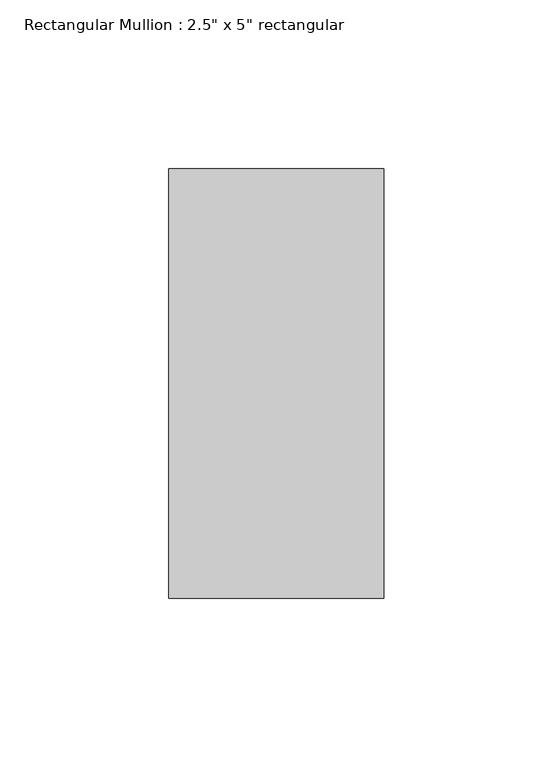
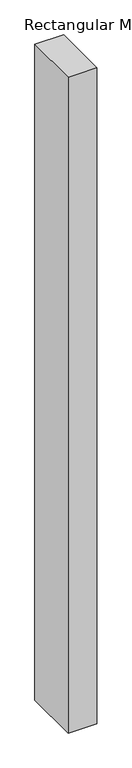
"""IFC4 building model written with IfcOpenShell, lengths in millimetres: member geometry."""

from ifc_helpers import new_model, si_unit, frame, origin, place, context, project, spatial, polyline, outline, extrude, source, transform, mapped, element, save


def member_6edf370a(model_context):
    return source(origin(), model_context, "Body", "SweptSolid", [
        extrude(outline(polyline([(0.0, 63.5), (0.0, -63.5), (-63.5, -63.5), (-63.5, 63.5), (0.0, 63.5)])), frame((0.0, 0.0, -1532.0284144), z_axis=(0.0, 0.0, 1.0), x_axis=(1.0, 0.0, 0.0)), (0.0, 0.0, 1.0), 1532.0284144),
    ])


if __name__ == "__main__":
    model = new_model("IFC4")
    model_context = context("Model", 3, world=origin())
    ifc_project = project(units=[si_unit("LENGTHUNIT", "METRE", prefix="MILLI")], contexts=[model_context])
    site = spatial("IfcSite", under=ifc_project)
    building = spatial("IfcBuilding", under=site)
    placement = place(None, origin())
    member_shape = member_6edf370a(model_context)
    element("IfcMember", 1, ObjectType="Rectangular Mullion : 2.5\" x 5\" rectangular", at=placement, inside=building, context=model_context, shape_type="MappedRepresentation", body=[
        mapped(member_shape, transform((0.0, 0.0, 0.0), x_axis=(1.0, 0.0, 0.0), y_axis=(0.0, 1.0, 0.0), z_axis=(0.0, 0.0, 1.0))),
    ])
    save(model, "model.ifc")

# Revit data of these elements
# Type "Rectangular Mullion : 2.5\" x 5\" rectangular"
#   built-in parameter 1007304 = 0.416667 (stored number, unit not read)
#   built-in parameter 1007301 = 0.104167 (stored number, unit not read)
#   built-in parameter 1007300 = 0.104167 (stored number, unit not read)
# Element 1 (IfcMember, "Rectangular Mullion : 2.5\" x 5\" rectangular")
#   Materials on its faces: "Aluminum"
# Materials
#   "Aluminum": class "Metal", colour RGB 247 247 247, transparency 0, Description = "Aluminum 6061", Cost = 0
